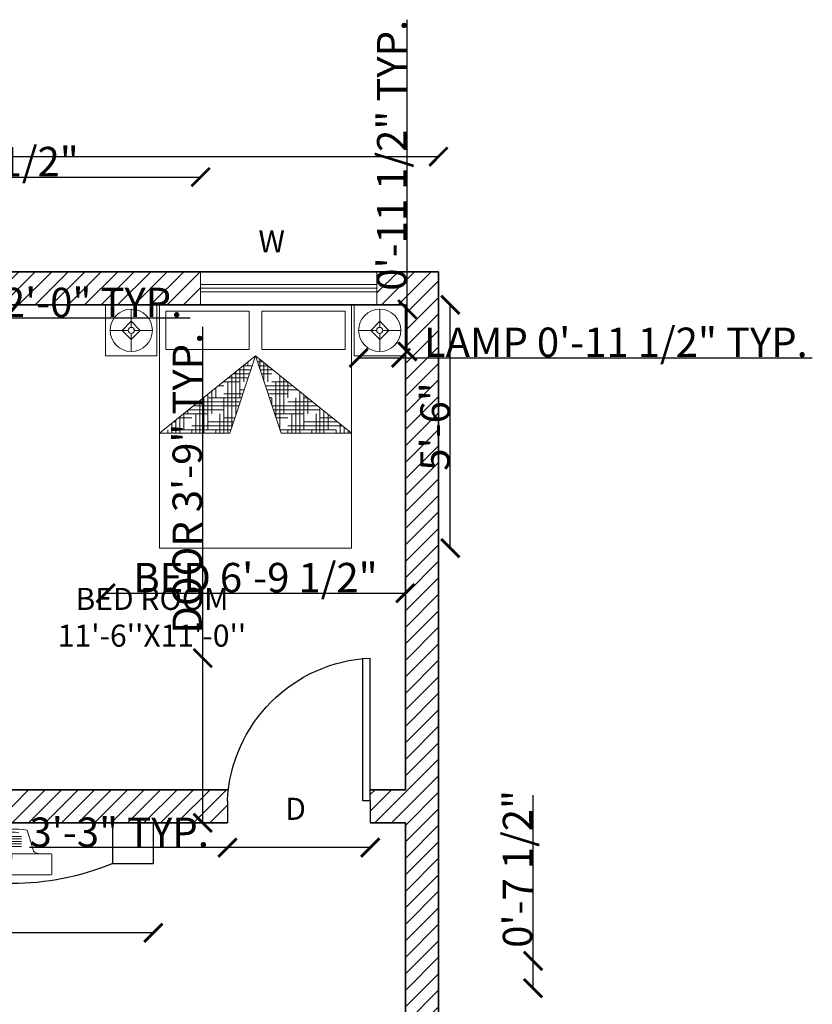
# Model space of a CAD drawing. Units: inches. Extents: x 2094 to 2639, y 1426 to 1997.
# Tile 8 of 8: x 2423 to 2639, y 1730 to 1997. Entities that reach past the tile are written whole.
import ezdxf

# ---------------------------------------------------------------- set-up
doc = ezdxf.new("R2010")
doc.units = ezdxf.units.IN
for name, color, linetype, lineweight in [('A-ANNO-DIMS', 2, 'Continuous', 18), ('A-ANNO-TEXT', 7, 'Continuous', 18), ('A-AREA-IDEN', 7, 'Continuous', 25), ('A-FURN', 8, 'Continuous', 18), ('A-WALL-PATT', 8, 'Continuous', 13), ('Doors', 34, 'Continuous', 25), ('Walls', 7, 'Continuous', 35), ('Windows', 150, 'Continuous', 18)]:
    doc.layers.add(name, color=color, linetype=linetype, lineweight=lineweight)
doc.layers.add('THIET-BI', color=21, linetype='Continuous')
doc.styles.get("Standard").update_dxf_attribs({"font": 'arial.ttf'})
doc.dimstyles.get("Standard").update_dxf_attribs({"dimtxt": 8, "dimasz": 5, "dimexe": 0.18, "dimexo": 0.0625, "dimgap": 0.09, "dimtad": 1, "dimdec": 1, "dimzin": 0, "dimdsep": 46, "dimlunit": 4, "dimtxsty": 'Standard', "dimblk": 'ARCHTICK', "dimcen": 0.09, "dimse1": 1, "dimse2": 1, "dimadec": 0, "dimazin": 0, "dimtfac": 1, "dimtdec": 1, "dimtofl": 0, "dimtmove": 0, "dimatfit": 3, "dimfxl": 1, "dimtolj": 1, "dimtzin": 0, "dimarcsym": 0})

# ---------------------------------------------------------------- blocks, each defined once
blk = doc.blocks.new('*X3')
at = {"color": 0}
for p, q in [((20.1875, 14.75), (20.1875, 14.7669)), ((20.199, 14.7812), (20.2772, 14.7812)), ((20.25, 14.8125), (20.2772, 14.8125)), ((20.1236, 14.6875), (20.25, 14.6875)), ((20.125, 14.5), (20.125, 14.6893)), ((20.1487, 14.7188), (20.2772, 14.7188)), ((20.1562, 14.625), (20.1562, 14.7281)), ((20.1739, 14.75), (20.2772, 14.75)), ((20.25, 14.3194), (20.25, 14.75)), ((20.0625, 14.2573), (20.0625, 14.6116)), ((20.0938, 14.375), (20.0938, 14.6504)), ((20.0984, 14.6562), (20.125, 14.6562)), ((20.2188, 14.3091), (20.2188, 14.625)), ((20.25, 14.625), (20.2772, 14.625)), ((19.9979, 14.5312), (20.2772, 14.5312)), ((20.023, 14.5625), (20.2772, 14.5625)), ((20.0312, 14.2469), (20.0312, 14.5727)), ((20.125, 14.5938), (20.2772, 14.5938)), ((19.9476, 14.4688), (20.125, 14.4688)), ((19.9727, 14.5), (20.25, 14.5)), ((20, 14.2366), (20, 14.5)), ((20.1875, 14.2987), (20.1875, 14.5)), ((19.875, 14.25), (19.875, 14.3785)), ((19.9062, 14.375), (19.9062, 14.4174)), ((19.9225, 14.4375), (20, 14.4375)), ((19.9688, 14.2262), (19.9688, 14.375)), ((20, 14.375), (20.2772, 14.375)), ((20.125, 14.4062), (20.2772, 14.4062)), ((20.1562, 14.2884), (20.1562, 14.375)), ((20.25, 14.4375), (20.2772, 14.4375)), ((19.8125, 14.1744), (19.8125, 14.3008)), ((19.8219, 14.3125), (20.2291, 14.3125)), ((19.8438, 14.1848), (19.8438, 14.3397)), ((19.875, 14.3438), (20.2772, 14.3438)), ((19.7465, 14.2188), (19.875, 14.2188)), ((19.75, 14.1537), (19.75, 14.2231)), ((19.7716, 14.25), (20, 14.25)), ((19.7812, 14.1641), (19.7812, 14.262)), ((19.7967, 14.2812), (20.125, 14.2812)), ((19.9375, 14.2159), (19.9375, 14.25)), ((19.7213, 14.1875), (19.75, 14.1875)), ((19.7018, 14.0938), (19.7786, 14.0938)), ((19.7188, 14.0726), (19.7188, 14.1136)), ((19.75, 14.0338), (19.75, 14.1032)), ((19.7812, 13.9949), (19.7812, 14.0929)), ((19.8125, 14), (19.8125, 14.0825)), ((19.7269, 14.0625), (19.8728, 14.0625)), ((19.752, 14.0312), (19.875, 14.0312)), ((19.875, 13.8784), (19.875, 14)), ((19.9062, 13.8396), (19.9062, 14.0514)), ((19.9375, 13.8007), (19.9375, 14.0411)), ((19.9688, 13.875), (19.9688, 14.0307)), ((20, 14), (20, 14.0204)), ((20, 14), (20.0614, 14)), ((20.0625, 13.6454), (20.0625, 13.9996)), ((20.0938, 13.625), (20.0938, 13.9893)), ((19.8275, 13.9375), (20.25, 13.9375)), ((19.875, 13.9688), (20.1557, 13.9688)), ((20.125, 13.75), (20.125, 13.9789)), ((20.1562, 13.875), (20.1562, 13.9686)), ((20.25, 13.5), (20.25, 13.9375)), ((19.8526, 13.9062), (20.125, 13.9062)), ((19.8777, 13.875), (20, 13.875)), ((20.0312, 13.6842), (20.0312, 13.875)), ((20.125, 13.8438), (20.2772, 13.8438)), ((20.2188, 13.4511), (20.2188, 13.875)), ((20.25, 13.875), (20.2772, 13.875)), ((19.9532, 13.7812), (20.2772, 13.7812)), ((20, 13.8125), (20.2772, 13.8125)), ((19.9783, 13.75), (20.25, 13.75)), ((20, 13.723), (20, 13.75)), ((20.0035, 13.7188), (20.125, 13.7188)), ((20.1875, 13.49), (20.1875, 13.75)), ((20.25, 13.6875), (20.2772, 13.6875)), ((20.0789, 13.625), (20.2772, 13.625)), ((20.125, 13.6562), (20.2772, 13.6562)), ((20.1562, 13.5288), (20.1562, 13.625)), ((20.104, 13.5938), (20.2772, 13.5938)), ((20.1292, 13.5625), (20.25, 13.5625)), ((20.2046, 13.4688), (20.2772, 13.4688)), ((20.25, 13.5), (20.2772, 13.5)), ((20.2297, 13.4375), (20.2772, 13.4375)), ((20.2549, 13.4062), (20.2772, 13.4062))]:
    blk.add_line(p, q, dxfattribs=at)
blk = doc.blocks.new('MAT-P13')
for p, q in [((-1.17, 0), (-1.17, -0.4)), ((-1.17, 0), (-0.77, 0)), ((-0.77, 0), (-0.77, -0.4)), ((-0.75, 0), (0.75, 0)), ((-0.75, 0), (-0.75, -1.9)), ((0.75, 0), (0.75, -1.9)), ((0.77, 0), (1.17, 0)), ((0.77, 0), (0.77, -0.4)), ((1.17, 0), (1.17, -0.4)), ((-0.7, -0.05), (-0.7, -0.35)), ((-0.7, -0.05), (-0.05, -0.05)), ((-0.05, -0.35), (-0.05, -0.05)), ((0.05, -0.05), (0.7, -0.05)), ((0.05, -0.35), (0.05, -0.05)), ((0.7, -0.05), (0.7, -0.35)), ((-0.7, -0.35), (-0.05, -0.35)), ((0.05, -0.35), (0.7, -0.35)), ((-1.17, -0.4), (-0.77, -0.4)), ((-0.75, -1.0034), (0, -0.4)), ((0, -0.4), (-0.75, -1.0034)), ((0, -0.4), (-0.2, -1.0034)), ((0, -0.4), (0.2, -1.0034)), ((0, -0.4), (0.75, -1.0034)), ((0.77, -0.4), (1.17, -0.4)), ((-0.75, -1.0034), (-0.2, -1.0034)), ((0.2, -1.0034), (0.75, -1.0034)), ((0.75, -1.9), (-0.75, -1.9))]:
    blk.add_line(p, q)
at = {"xscale": -1, "rotation": 90}
blk.add_blockref('*X3', (14.1285, 19.2738), dxfattribs=at)
blk = doc.blocks.new('Lamp - Table')
for p, q in [((0, 7), (0, 1)), ((-1, 0), (-7, 0)), ((0, 3), (-3, 0)), ((-3, 0), (0, -3)), ((3, 0), (0, 3)), ((0, -3), (3, 0)), ((1, 0), (7, 0)), ((0, -1), (0, -7))]:
    blk.add_line(p, q)
for radius in [7, 1]:
    blk.add_circle((0, 0), radius)
blk = doc.blocks.new('TVI01')
for p, q in [((-155.1, -10), (-213, -204.9)), ((-97.7, -72.9), (99, -72.9)), ((155.1, -10), (214.2, -208.9)), ((-97.7, -97.9), (99, -97.9)), ((-97.7, -122.9), (99, -122.9)), ((-97.7, -146.1), (99, -146.1)), ((-97.7, -172.9), (99, -172.9)), ((-400, -254.3), (-400, -441.4)), ((-391.8, -243.8), (391.8, -243.8)), ((-3.8, -247.8), (4.2, -432.2)), ((4.2, -247.8), (10.5, -243.6)), ((4.2, -247.8), (130.6, -471.4)), ((4.2, -247.8), (4.2, -432.2)), ((10.5, -243.6), (130.6, -471.4)), ((400, -254.3), (400, -441.4)), ((-391.8, -451.9), (391.8, -451.9))]:
    blk.add_line(p, q)
for centre, radius, start, end in [((0, -1207.7), 1207.7, 82.62163, 97.37837), ((0, -325), 295, 75.74997, 104.25003), ((-390, -253.7), 10, 100.35421, 183.7314), ((-75.1, -1338.2), 1112.5, 99.19763, 100.35421), ((-260.9, -190.6), 50, 279.19763, 343.45736), ((0.2, -247.8), 4, 0, 184.96916), ((260.9, -190.6), 50, 196.54264, 260.80237), ((75.1, -1338.2), 1112.5, 79.64579, 80.80237), ((390, -253.7), 10, 356.2686, 100.69826), ((-390, -442), 10, 176.2686, 259.64579), ((390, -442), 10, 280.35421, 3.7314)]:
    blk.add_arc(centre, radius, start, end)
blk = doc.blocks.new('A$C4C711776')
at = {"layer": 'THIET-BI'}
for p, q in [((180, 2160), (180, 2520)), ((180, 2520), (540, 2520)), ((540, 2160), (180, 2160)), ((180, 360), (180, 0)), ((180, 360), (540, 360)), ((180, 0), (540, 0))]:
    blk.add_line(p, q, dxfattribs=at)
at = {"layer": 'THIET-BI', "extrusion": (0, 0, -1)}
blk.add_ellipse((2340, 1260), major_axis=(1654.6, 1654.6), ratio=1, start_param=3.5322, end_param=4.321782, dxfattribs=at)
at = {"color": 0, "extrusion": (0, 0, -1), "xscale": 0.9000000000014551, "yscale": 0.9000000000014551, "zscale": -0.9, "rotation": 90}
blk.add_blockref('TVI01', (-485.3, 1261.3), dxfattribs=at)
blk = doc.blocks.new('AP0B05')
for p, q in [((35, 100), (35, 880)), ((75, 100), (75, 878.9)), ((35, 100), (35, -20)), ((815, 100), (815, -20))]:
    blk.add_line(p, q)
blk.add_lwpolyline([(35, 100), (75, 100)])
blk.add_arc((-2.4, 62.6), 818.3, 2.6212, 87.3788)
blk = doc.blocks.new('_ArchTick')
at = {"color": 0, "linetype": 'ByBlock', "const_width": 0.15}
blk.add_lwpolyline([(-0.5, -0.5), (0.5, 0.5)], dxfattribs=at)
blk = doc.blocks.new('*D13')
at = {"layer": 'A-ANNO-DIMS', "color": 0, "lineweight": -2, "transparency": 16777216}
blk.add_line((2180.06, 1960.22), (2537.06, 1960.22), dxfattribs=at)
at = {"layer": 'Defpoints', "color": 0, "transparency": 16777216}
for p in [(2537.06, 1960.22), (2180.06, 1928.9), (2537.06, 1928.9)]:
    blk.add_point(p, dxfattribs=at)
at = {"layer": 'A-ANNO-DIMS', "color": 0, "lineweight": -2, "transparency": 16777216, "xscale": 5, "yscale": 5, "zscale": 5, "rotation": 180}
blk.add_blockref('_ArchTick', (2180.06, 1960.22), dxfattribs=at)
at = {"layer": 'A-ANNO-DIMS', "color": 0, "lineweight": -2, "transparency": 16777216, "xscale": 5, "yscale": 5, "zscale": 5}
blk.add_blockref('_ArchTick', (2537.06, 1960.22), dxfattribs=at)
at = {"layer": 'A-ANNO-DIMS', "color": 0, "transparency": 16777216, "insert": (2358.56, 1964.39), "char_height": 8, "attachment_point": 5}
blk.add_mtext('\\A1;29\'-9"', dxfattribs=at)
blk = doc.blocks.new('WIN-48IN')
for p, q in [((0, 5.5), (48, 5.5)), ((0, 4.5), (48, 4.5)), ((0, 3.5), (48, 3.5))]:
    blk.add_line(p, q)
blk.add_lwpolyline([(0, 0), (48, 0), (48, 9), (0, 9)], close=True)
blk = doc.blocks.new('*D21')
at = {"layer": 'A-ANNO-DIMS', "color": 0, "lineweight": -2, "transparency": 16777216}
for p, q in [((2472.91, 1823.73), (2472.91, 1913.91)), ((2472.91, 1778.9), (2472.91, 1823.73))]:
    blk.add_line(p, q, dxfattribs=at)
at = {"layer": 'Defpoints', "color": 0, "transparency": 16777216}
for p in [(2472.91, 1823.73), (2479.64, 1823.73), (2479.64, 1778.9)]:
    blk.add_point(p, dxfattribs=at)
at = {"layer": 'A-ANNO-DIMS', "color": 0, "lineweight": -2, "transparency": 16777216, "xscale": 5, "yscale": 5, "zscale": 5}
for p, rotation in [((2472.91, 1823.73), 90), ((2472.91, 1778.9), 270)]:
    blk.add_blockref('_ArchTick', p, dxfattribs=dict(at, rotation=rotation))
at = {"layer": 'A-ANNO-DIMS', "color": 0, "transparency": 16777216, "insert": (2468.68, 1871.32), "char_height": 8, "attachment_point": 5, "rotation": 90}
blk.add_mtext('\\A1;DOOR 3\'-9" TYP.', dxfattribs=at)
blk = doc.blocks.new('*D22')
at = {"layer": 'A-ANNO-DIMS', "color": 0, "lineweight": -2, "transparency": 16777216}
for p, q in [((2479.64, 1772.17), (2425.7, 1772.17)), ((2518.5, 1772.17), (2479.64, 1772.17))]:
    blk.add_line(p, q, dxfattribs=at)
at = {"layer": 'Defpoints', "color": 0, "transparency": 16777216}
for p in [(2479.64, 1778.9), (2518.5, 1778.9), (2479.64, 1772.17)]:
    blk.add_point(p, dxfattribs=at)
at = {"layer": 'A-ANNO-DIMS', "color": 0, "lineweight": -2, "transparency": 16777216, "xscale": 5, "yscale": 5, "zscale": 5, "rotation": 180}
blk.add_blockref('_ArchTick', (2479.64, 1772.17), dxfattribs=at)
at = {"layer": 'A-ANNO-DIMS', "color": 0, "lineweight": -2, "transparency": 16777216, "xscale": 5, "yscale": 5, "zscale": 5}
blk.add_blockref('_ArchTick', (2518.5, 1772.17), dxfattribs=at)
at = {"layer": 'A-ANNO-DIMS', "color": 0, "transparency": 16777216, "insert": (2450.17, 1776.35), "char_height": 8, "attachment_point": 5}
blk.add_mtext('\\A1;3\'-3" TYP.', dxfattribs=at)
blk = doc.blocks.new('*D29')
at = {"layer": 'A-ANNO-DIMS', "color": 0, "lineweight": -2, "transparency": 16777216}
for p, q in [((2339.06, 1916.3), (2363.06, 1916.3)), ((2363.06, 1916.3), (2469.47, 1916.3))]:
    blk.add_line(p, q, dxfattribs=at)
at = {"layer": 'Defpoints', "color": 0, "transparency": 16777216}
for p in [(2339.06, 1919.9), (2363.06, 1919.9), (2363.06, 1916.3)]:
    blk.add_point(p, dxfattribs=at)
at = {"layer": 'A-ANNO-DIMS', "color": 0, "lineweight": -2, "transparency": 16777216, "xscale": 5, "yscale": 5, "zscale": 5, "rotation": 180}
blk.add_blockref('_ArchTick', (2339.06, 1916.3), dxfattribs=at)
at = {"layer": 'A-ANNO-DIMS', "color": 0, "lineweight": -2, "transparency": 16777216, "xscale": 5, "yscale": 5, "zscale": 5}
blk.add_blockref('_ArchTick', (2363.06, 1916.3), dxfattribs=at)
at = {"layer": 'A-ANNO-DIMS', "color": 0, "transparency": 16777216, "insert": (2418.76, 1920.53), "char_height": 8, "attachment_point": 5}
blk.add_mtext('\\A1;WINDOW 2\'-0" TYP.', dxfattribs=at)
blk = doc.blocks.new('*D31')
at = {"layer": 'A-ANNO-DIMS', "color": 0, "lineweight": -2, "transparency": 16777216}
blk.add_line((2446.47, 1841.41), (2528.06, 1841.41), dxfattribs=at)
at = {"layer": 'Defpoints', "color": 0, "transparency": 16777216}
for p in [(2446.47, 1853.65), (2528.06, 1853.65), (2528.06, 1841.41)]:
    blk.add_point(p, dxfattribs=at)
at = {"layer": 'A-ANNO-DIMS', "color": 0, "lineweight": -2, "transparency": 16777216, "xscale": 5, "yscale": 5, "zscale": 5, "rotation": 180}
blk.add_blockref('_ArchTick', (2446.47, 1841.41), dxfattribs=at)
at = {"layer": 'A-ANNO-DIMS', "color": 0, "lineweight": -2, "transparency": 16777216, "xscale": 5, "yscale": 5, "zscale": 5}
blk.add_blockref('_ArchTick', (2528.06, 1841.41), dxfattribs=at)
at = {"layer": 'A-ANNO-DIMS', "color": 0, "transparency": 16777216, "insert": (2487.26, 1845.64), "char_height": 8, "attachment_point": 5}
blk.add_mtext('\\A1;BED 6\'-9 1/2"', dxfattribs=at)
blk = doc.blocks.new('*D32')
at = {"layer": 'A-ANNO-DIMS', "color": 0, "lineweight": -2, "transparency": 16777216}
blk.add_line((2540.29, 1853.65), (2540.29, 1919.9), dxfattribs=at)
at = {"layer": 'Defpoints', "color": 0, "transparency": 16777216}
for p in [(2528.06, 1919.9), (2540.29, 1919.9), (2528.06, 1853.65)]:
    blk.add_point(p, dxfattribs=at)
at = {"layer": 'A-ANNO-DIMS', "color": 0, "lineweight": -2, "transparency": 16777216, "xscale": 5, "yscale": 5, "zscale": 5}
for p, rotation in [((2540.29, 1919.9), 90), ((2540.29, 1853.65), 270)]:
    blk.add_blockref('_ArchTick', p, dxfattribs=dict(at, rotation=rotation))
at = {"layer": 'A-ANNO-DIMS', "color": 0, "transparency": 16777216, "insert": (2536.12, 1886.77), "char_height": 8, "attachment_point": 5, "rotation": 90}
blk.add_mtext('\\A1;5\'-6"', dxfattribs=at)
blk = doc.blocks.new('*D35')
at = {"layer": 'A-ANNO-DIMS', "color": 0, "lineweight": -2, "transparency": 16777216}
for p, q in [((2515.33, 1905.45), (2526.83, 1905.45)), ((2526.83, 1905.45), (2638.82, 1905.45))]:
    blk.add_line(p, q, dxfattribs=at)
at = {"layer": 'Defpoints', "color": 0, "transparency": 16777216}
for p in [(2515.33, 1907.18), (2526.83, 1907.18), (2526.83, 1905.45)]:
    blk.add_point(p, dxfattribs=at)
at = {"layer": 'A-ANNO-DIMS', "color": 0, "lineweight": -2, "transparency": 16777216, "xscale": 5, "yscale": 5, "zscale": 5, "rotation": 180}
blk.add_blockref('_ArchTick', (2515.33, 1905.45), dxfattribs=at)
at = {"layer": 'A-ANNO-DIMS', "color": 0, "lineweight": -2, "transparency": 16777216, "xscale": 5, "yscale": 5, "zscale": 5}
blk.add_blockref('_ArchTick', (2526.83, 1905.45), dxfattribs=at)
at = {"layer": 'A-ANNO-DIMS', "color": 0, "transparency": 16777216, "insert": (2585.33, 1909.68), "char_height": 8, "attachment_point": 5}
blk.add_mtext('\\A1;LAMP 0\'-11 1/2" TYP.', dxfattribs=at)
blk = doc.blocks.new('*D36')
at = {"layer": 'A-ANNO-DIMS', "color": 0, "lineweight": -2, "transparency": 16777216}
for p, q in [((2528.56, 1918.68), (2528.56, 1997.48)), ((2528.56, 1907.18), (2528.56, 1918.68))]:
    blk.add_line(p, q, dxfattribs=at)
at = {"layer": 'Defpoints', "color": 0, "transparency": 16777216}
for p in [(2526.83, 1918.68), (2528.56, 1918.68), (2526.83, 1907.18)]:
    blk.add_point(p, dxfattribs=at)
at = {"layer": 'A-ANNO-DIMS', "color": 0, "lineweight": -2, "transparency": 16777216, "xscale": 5, "yscale": 5, "zscale": 5}
for p, rotation in [((2528.56, 1918.68), 90), ((2528.56, 1907.18), 270)]:
    blk.add_blockref('_ArchTick', p, dxfattribs=dict(at, rotation=rotation))
at = {"layer": 'A-ANNO-DIMS', "color": 0, "transparency": 16777216, "insert": (2524.33, 1960.58), "char_height": 8, "attachment_point": 5, "rotation": 90}
blk.add_mtext('\\A1;0\'-11 1/2" TYP.', dxfattribs=at)
blk = doc.blocks.new('*D49')
at = {"layer": 'A-ANNO-DIMS', "color": 0, "lineweight": -2, "transparency": 16777216}
for p, q in [((2382.28, 1748.95), (2288.52, 1748.95)), ((2459.46, 1748.95), (2382.28, 1748.95))]:
    blk.add_line(p, q, dxfattribs=at)
at = {"layer": 'Defpoints', "color": 0, "transparency": 16777216}
for p in [(2382.28, 1760.52), (2459.46, 1760.52), (2382.28, 1748.95)]:
    blk.add_point(p, dxfattribs=at)
at = {"layer": 'A-ANNO-DIMS', "color": 0, "lineweight": -2, "transparency": 16777216, "xscale": 5, "yscale": 5, "zscale": 5, "rotation": 180}
blk.add_blockref('_ArchTick', (2382.28, 1748.95), dxfattribs=at)
at = {"layer": 'A-ANNO-DIMS', "color": 0, "lineweight": -2, "transparency": 16777216, "xscale": 5, "yscale": 5, "zscale": 5}
blk.add_blockref('_ArchTick', (2459.46, 1748.95), dxfattribs=at)
at = {"layer": 'A-ANNO-DIMS', "color": 0, "transparency": 16777216, "insert": (2332.9, 1753.12), "char_height": 8, "attachment_point": 5}
blk.add_mtext('\\A1;MEDIA UNIT 6\'-5"', dxfattribs=at)
blk = doc.blocks.new('*D55')
at = {"layer": 'A-ANNO-DIMS', "color": 0, "lineweight": -2, "transparency": 16777216}
blk.add_line((2363.06, 1954.65), (2472.33, 1954.65), dxfattribs=at)
at = {"layer": 'Defpoints', "color": 0, "transparency": 16777216}
for p in [(2472.33, 1954.65), (2363.06, 1928.9), (2472.33, 1928.9)]:
    blk.add_point(p, dxfattribs=at)
at = {"layer": 'A-ANNO-DIMS', "color": 0, "lineweight": -2, "transparency": 16777216, "xscale": 5, "yscale": 5, "zscale": 5, "rotation": 180}
blk.add_blockref('_ArchTick', (2363.06, 1954.65), dxfattribs=at)
at = {"layer": 'A-ANNO-DIMS', "color": 0, "lineweight": -2, "transparency": 16777216, "xscale": 5, "yscale": 5, "zscale": 5}
blk.add_blockref('_ArchTick', (2472.33, 1954.65), dxfattribs=at)
at = {"layer": 'A-ANNO-DIMS', "color": 0, "transparency": 16777216, "insert": (2417.69, 1958.87), "char_height": 8, "attachment_point": 5}
blk.add_mtext('\\A1;9\'-1 1/2"', dxfattribs=at)
blk = doc.blocks.new('*D79')
at = {"layer": 'A-ANNO-DIMS', "color": 0, "lineweight": -2, "transparency": 16777216}
for p, q in [((2562.81, 1741.32), (2562.81, 1786.41)), ((2562.81, 1733.9), (2562.81, 1741.32))]:
    blk.add_line(p, q, dxfattribs=at)
at = {"layer": 'Defpoints', "color": 0, "transparency": 16777216}
for p in [(2309.06, 1741.32), (2562.81, 1741.32), (2309.06, 1733.9)]:
    blk.add_point(p, dxfattribs=at)
at = {"layer": 'A-ANNO-DIMS', "color": 0, "lineweight": -2, "transparency": 16777216, "xscale": 5, "yscale": 5, "zscale": 5}
for p, rotation in [((2562.81, 1741.32), 90), ((2562.81, 1733.9), 270)]:
    blk.add_blockref('_ArchTick', p, dxfattribs=dict(at, rotation=rotation))
at = {"layer": 'A-ANNO-DIMS', "color": 0, "transparency": 16777216, "insert": (2558.58, 1766.37), "char_height": 8, "attachment_point": 5, "rotation": 90}
blk.add_mtext('\\A1;0\'-7 1/2"', dxfattribs=at)

msp = doc.modelspace()

# ---------------------------------------------------------------- hatches: boundary and pattern name
at = {"layer": 'A-WALL-PATT', "transparency": 33554585}
h = msp.add_hatch(dxfattribs=at)
h.set_pattern_fill('ANSI31', color=256)
h.paths.add_polyline_path([(2189.06, 1727.9), (2230.3, 1727.9, -0.022928), (2230.09, 1730.2), (2230.09, 1733.9), (2189.06, 1733.9), (2189.06, 1742.37), (2180.06, 1742.37), (2180.06, 1714.4), (2189.06, 1714.4)])
h.paths.add_polyline_path([(2456.51, 1574.9), (2413.83, 1574.9), (2413.83, 1565.9), (2456.51, 1565.9)])
h.paths.add_polyline_path([(2537.06, 1643.81), (2528.06, 1643.81), (2528.06, 1574.9), (2519.78, 1574.9), (2519.78, 1571.88), (2519.78, 1565.9), (2537.06, 1565.9)])
h.paths.add_polyline_path([(2339.06, 1928.9), (2300.94, 1928.9), (2300.94, 1919.9), (2309.06, 1919.9), (2309.06, 1776.3, -0.024186), (2312.62, 1776.64), (2318.06, 1776.64), (2318.06, 1778.9), (2336.06, 1778.9), (2336.06, 1787.9), (2318.06, 1787.9), (2318.06, 1835.9), (2384.06, 1835.9), (2384.06, 1787.9), (2366.06, 1787.9), (2366.06, 1778.9), (2479.64, 1778.9), (2479.64, 1784.88, -0.018603), (2479.89, 1787.9), (2390.06, 1787.9), (2390.06, 1847.57), (2385.61, 1847.57), (2384.06, 1847.57), (2384.06, 1841.9), (2318.06, 1841.9), (2318.06, 1919.9), (2339.06, 1919.9)])
h.paths.add_polyline_path([(2252.94, 1928.9), (2180.06, 1928.9), (2180.06, 1790.37), (2189.06, 1790.37), (2189.06, 1843.77), (2189.06, 1919.9), (2252.94, 1919.9)])
h.paths.add_polyline_path([(2472.33, 1928.9), (2363.06, 1928.9), (2363.06, 1919.9), (2384.06, 1919.9), (2384.06, 1876.38, -0.012802), (2385.61, 1876.49), (2390.06, 1876.49), (2390.06, 1919.9), (2472.33, 1919.9)], flags=17)
h.paths.add_polyline_path([(2537.06, 1928.9), (2520.33, 1928.9), (2520.33, 1919.9), (2528.06, 1919.9), (2528.06, 1905.95), (2528.06, 1787.9), (2518.5, 1787.9), (2518.5, 1784.88), (2518.5, 1778.9), (2528.06, 1778.9), (2528.06, 1715.81), (2537.06, 1715.81)])
h.paths.add_polyline_path([(2379.33, 1857.12), (2393.06, 1857.12), (2393.06, 1866.16), (2379.33, 1866.16)], flags=25)
h.paths.add_polyline_path([(2235.85, 1725.77), (2249.57, 1725.77), (2249.57, 1734.81), (2235.85, 1734.81)], flags=25)
h.paths.add_polyline_path([(2305.79, 1754.6), (2314.84, 1754.6), (2314.84, 1763.6), (2305.79, 1763.6)], flags=9)
h.paths.add_polyline_path([(2493.85, 1778.22), (2502.9, 1778.22), (2502.9, 1787.22), (2493.85, 1787.22)], flags=9)
h.paths.add_polyline_path([(2370.69, 1555.65), (2381.6, 1555.65), (2381.6, 1564.65), (2370.69, 1564.65)], flags=9)
h.paths.add_polyline_path([(2461.57, 1555.65), (2477.6, 1555.65), (2477.6, 1564.65), (2461.57, 1564.65)], flags=9)
h.paths.add_polyline_path([(2493.18, 1565.15), (2509.22, 1565.15), (2509.22, 1574.15), (2493.18, 1574.15)], flags=9)
h.paths.add_polyline_path([(2408.32, 1501.7), (2449.12, 1501.7), (2449.12, 1520.36), (2408.32, 1520.36)], flags=9)
h.paths.add_polyline_path([(2398.49, 1698.6), (2441.61, 1698.6), (2441.61, 1717.26), (2398.49, 1717.26)], flags=9)
h.paths.add_polyline_path([(2248.63, 1683.29), (2287.87, 1683.29), (2287.87, 1701.95), (2248.63, 1701.95)], flags=25)
h.paths.add_polyline_path([(2440.73, 1823.2), (2483.86, 1823.2), (2483.86, 1841.85), (2440.73, 1841.85)], flags=9)
h.paths.add_polyline_path([(2335.3, 1804.5), (2370.65, 1804.5), (2370.65, 1823.15), (2335.3, 1823.15)], flags=25)
h.paths.add_polyline_path([(2335.3, 1893.12), (2370.65, 1893.12), (2370.65, 1911.77), (2335.3, 1911.77)], flags=25)
h.paths.add_polyline_path([(2241.82, 1863.6), (2290.11, 1863.6), (2290.11, 1882.25), (2241.82, 1882.25)], flags=9)

# ---------------------------------------------------------------- linework, layer by layer
at = {"layer": 'Walls'}
for p, q in [((2180.06, 1928.9), (2537.06, 1928.9)), ((2537.06, 1928.9), (2537.06, 1565.9)), ((2390.06, 1919.9), (2528.06, 1919.9)), ((2528.06, 1919.9), (2528.06, 1787.9)), ((2390.06, 1787.9), (2479.89, 1787.9)), ((2518.5, 1787.9), (2528.06, 1787.9)), ((2366.06, 1778.9), (2479.64, 1778.9)), ((2518.5, 1778.9), (2528.06, 1778.9)), ((2528.06, 1778.9), (2528.06, 1574.9))]:
    msp.add_line(p, q, dxfattribs=at)

# ---------------------------------------------------------------- block references
at = {"layer": 'A-FURN'}
for name, p, xscale, yscale, zscale in [('MAT-P13', (2487.26, 1919.9), 34.86719180358278, 34.86719180358278, 34.86719180358278), ('Lamp - Table', (2453.44, 1912.93), 0.8214292055513094, 0.8214292055513094, 0.8214292055513094), ('Lamp - Table', (2521.08, 1912.93), 0.8214292055513094, 0.8214292055513094, 0.8214292055513094)]:
    msp.add_blockref(name, p, dxfattribs=dict(at, xscale=xscale, yscale=yscale, zscale=zscale))
at = {"layer": 'A-FURN', "xscale": 0.0306262109582552, "yscale": 0.0306262109582552, "zscale": 0.0306262109582552, "rotation": 89.99999999999991}
msp.add_blockref('A$C4C711776', (2459.46, 1762.36), dxfattribs=at)
at = {"layer": 'Doors', "xscale": -0.0498171271707621, "yscale": 0.0498171271707621, "zscale": 0.0498171271707621}
msp.add_blockref('AP0B05', (2520.24, 1779.89), dxfattribs=at)
at = {"layer": 'Windows'}
msp.add_blockref('WIN-48IN', (2472.33, 1919.9), dxfattribs=at)

# ---------------------------------------------------------------- texts
at = {"layer": 'A-ANNO-TEXT'}
for s, p in [('W', (2488.07, 1934.12)), ('D', (2495.35, 1779.72))]:
    msp.add_text(s, height=6, dxfattribs=at).set_placement(p)
at = {"layer": 'A-AREA-IDEN', "insert": (2432.54, 1842.85), "char_height": 6, "attachment_point": 1}
msp.add_mtext_dynamic_manual_height_columns("\\pxqc;BED ROOM\\P11'-6''X11'-0''", width=53.0999, gutter_width=63.55, heights=[0], dxfattribs=at)

# ---------------------------------------------------------------- dimensions: what is measured, and where the dimension line sits
at = {"layer": 'A-ANNO-DIMS'}
for base, p1, p2, angle, text, picture, middle in [((2528.56, 1918.68), (2526.83, 1907.18), (2526.83, 1918.68), 90, '<> TYP.', '*D36', (2524.33, 1960.58)), ((2472.91, 1823.73), (2479.64, 1778.9), (2479.64, 1823.73), 90, 'DOOR <> TYP.', '*D21', (2468.68, 1871.32)), ((2479.64, 1772.17), (2518.5, 1778.9), (2479.64, 1778.9), 180, '<> TYP.', '*D22', (2450.17, 1776.35)), ((2382.28, 1748.95), (2459.46, 1760.52), (2382.28, 1760.52), 180, 'MEDIA UNIT <>', '*D49', (2332.9, 1753.12))]:
    dim = msp.add_linear_dim(base=base, p1=p1, p2=p2, angle=angle, text=text, dimstyle='Standard', override={"dimdec": 1, "dimlfac": 1, "dimrnd": 0, "dimzin": 1, "dimdsep": 46, "dimlunit": 4, "dimfrac": 2}, dxfattribs=at)
    dim.commit()
    dim.dimension.update_dxf_attribs({"geometry": picture, "text_midpoint": middle})
for base, p1, p2, override, picture, middle in [((2537.06, 1960.22), (2180.06, 1928.9), (2537.06, 1928.9), {"dimclrd": 0, "dimclre": 0, "dimclrt": 0}, '*D13', (2358.56, 1964.39)), ((2472.33, 1954.65), (2363.06, 1928.9), (2472.33, 1928.9), {"dimdec": 1, "dimlfac": 1, "dimrnd": 0, "dimzin": 1, "dimdsep": 46, "dimlunit": 4, "dimfrac": 2}, '*D55', (2417.69, 1958.87))]:
    dim = msp.add_linear_dim(base=base, p1=p1, p2=p2, dimstyle='Standard', override=override, dxfattribs=at)
    dim.commit()
    dim.dimension.update_dxf_attribs({"geometry": picture, "text_midpoint": middle})
for base, p1, p2, text, picture, middle in [((2363.06, 1916.3), (2339.06, 1919.9), (2363.06, 1919.9), 'WINDOW <> TYP.', '*D29', (2418.76, 1920.53)), ((2526.83, 1905.45), (2515.33, 1907.18), (2526.83, 1907.18), 'LAMP <> TYP.', '*D35', (2585.33, 1909.68)), ((2528.06, 1841.41), (2446.47, 1853.65), (2528.06, 1853.65), 'BED <>', '*D31', (2487.26, 1845.64))]:
    dim = msp.add_linear_dim(base=base, p1=p1, p2=p2, text=text, dimstyle='Standard', override={"dimdec": 1, "dimlfac": 1, "dimrnd": 0, "dimzin": 1, "dimdsep": 46, "dimlunit": 4, "dimfrac": 2}, dxfattribs=at)
    dim.commit()
    dim.dimension.update_dxf_attribs({"geometry": picture, "text_midpoint": middle})
for base, p1, p2, picture, middle in [((2540.2947, 1919.8985), (2528.0563, 1853.6509), (2528.0563, 1919.8985), '*D32', (2536.1201, 1886.7747)), ((2562.81, 1741.32), (2309.06, 1733.9), (2309.06, 1741.32), '*D79', (2558.58, 1766.37))]:
    dim = msp.add_linear_dim(base=base, p1=p1, p2=p2, angle=90, dimstyle='Standard', override={"dimdec": 1, "dimlfac": 1, "dimrnd": 0, "dimzin": 1, "dimdsep": 46, "dimlunit": 4, "dimfrac": 2}, dxfattribs=at)
    dim.commit()
    dim.dimension.update_dxf_attribs({"geometry": picture, "text_midpoint": middle})

doc.saveas('drawing.dxf')
